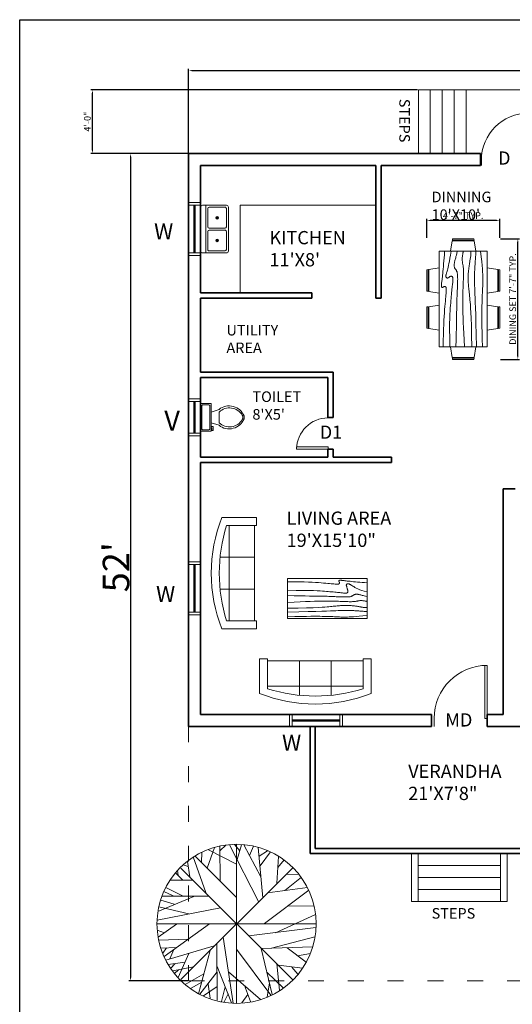
# Model space of a CAD drawing. Units: inches. Extents: x 1662 to 23131, y 1265 to 19127.
# Tile 24 of 26: x 21861 to 22232, y 18361 to 19104. Entities that reach past the tile are written whole.
import ezdxf

# ---------------------------------------------------------------- set-up
doc = ezdxf.new("R2010")
doc.units = ezdxf.units.IN
doc.linetypes.add('ACAD_ISO03W100', pattern=[30, 12, -18])
for name, color, linetype, lineweight in [('A-ANNO-DIMS', 4, 'Continuous', 18), ('A-ANNO-IDEN', 7, 'Continuous', 18), ('A-ANNO-TTLB', 7, 'Continuous', 25), ('A-AREA-IDEN', 7, 'Continuous', 18), ('A-DOOR', 3, 'Continuous', 18), ('A-FLOR-CASE', 8, 'Continuous', 18), ('A-FLOR-FIXT', 9, 'Continuous', 18), ('A-FLOR-STRS', 7, 'Continuous', 18), ('A-FURN', 8, 'Continuous', 18), ('A-GLAZ', 4, 'Continuous', 18), ('A-SITE-PRKG', 8, 'ACAD_ISO03W100', 18), ('A-WALL', 7, 'Continuous', 35), ('L-PLNT', 3, 'Continuous', 18)]:
    doc.layers.add(name, color=color, linetype=linetype, lineweight=lineweight)
doc.styles.get("Standard").update_dxf_attribs({"font": 'arial.ttf'})
doc.dimstyles.new('ISO-25', dxfattribs={"dimtxt": 5, "dimasz": 2.5, "dimexe": 1.25, "dimexo": 0.625, "dimtad": 1, "dimlunit": 3, "dimtxsty": 'Standard', "dimcen": 2.5, "dimadec": 0, "dimazin": 0, "dimtfac": 1, "dimtmove": 0, "dimatfit": 3, "dimfxl": 1, "dimarcsym": 0})

# ---------------------------------------------------------------- blocks, each defined once
blk = doc.blocks.new('*U27')
for p, q in [((0, 0), (0, -6)), ((-40, 0), (-40, -6))]:
    blk.add_line(p, q)
blk.add_lwpolyline([(0, 0), (0, 40), (-1.75, 40), (-1.75, 0)], close=True)
blk.add_arc((0, 0), 40, 90, 180)
blk = doc.blocks.new('*U119')
for p, q in [((-600, 0), (-600, 100)), ((0, 0), (0, 100))]:
    blk.add_line(p, q)
blk.add_lwpolyline([(0, 0), (0, -600), (-43.75, -600), (-43.75, 0)], close=True)
blk.add_arc((0, 0), 600, 180, 270)
blk = doc.blocks.new('*U121')
for p, q in [((0, 0), (0, -100)), ((-900, 0), (-900, -100))]:
    blk.add_line(p, q)
blk.add_lwpolyline([(0, 0), (0, 900), (-43.75, 900), (-43.75, 0)], close=True)
blk.add_arc((0, 0), 900, 90, 180)
blk = doc.blocks.new('Toilet - top')
for p, q in [((9.5, -6), (9.5, -2)), ((-10, -8.5), (-8, -8.5)), ((-10, -9.5), (-10, -8.5)), ((-7, -9.5), (-10, -9.5)), ((-8, -8.5), (-8, -8)), ((-7, -8), (-7, -9.5)), ((-4, -8), (-6, -14)), ((4, -14), (-4, -14)), ((4, -8), (6, -14))]:
    blk.add_line(p, q)
blk.add_lwpolyline([(10.5, -8), (10.5, 0), (-10.5, 0), (-10.5, -8)], close=True)
for points in [[(-9.5, -2), (-9.5, -6)], [(8.5, -1), (-8.5, -1)], [(-8.5, -7), (8.5, -7)]]:
    blk.add_lwpolyline(points)
for centre, radius, start, end in [((-8.62, -1.88), 0.884, 81.8699, 188.1301), ((-8.62, -6.12), 0.884, 171.8699, 278.1301), ((8.62, -1.88), 0.884, 351.8699, 98.1301), ((8.62, -6.12), 0.884, 261.8699, 8.1301), ((3.52, -21.58), 12.17, 141.46911, 247.97143), ((4.2, -21.82), 11.33, 136.36773, 238.94682), ((-3.52, -21.58), 12.17, 292.02843, 38.53071), ((-4.2, -21.82), 11.33, 301.05301, 43.63209), ((0, -27.88), 4, 245.73182, 294.26817), ((0, -29), 4, 254.86053, 285.13947)]:
    blk.add_arc(centre, radius, start, end)
blk = doc.blocks.new('Sink-double - 36 in top')
for p, q in [((-18, -4), (18, -4)), ((-0.75, -18.5), (-0.75, -6.5)), ((0.75, -6.5), (0.75, -18.5))]:
    blk.add_line(p, q)
for points in [[(-16.5, 0), (16.5, 0)], [(-18, -19.5), (-18, -1.5)], [(-16.5, -18.5), (-16.5, -6.5)], [(-15.5, -5.5), (-1.75, -5.5)], [(1.75, -5.5), (15.5, -5.5)], [(16.5, -6.5), (16.5, -18.5)], [(18, -1.5), (18, -19.5)], [(16.5, -21), (-16.5, -21)], [(-1.75, -19.5), (-15.5, -19.5)], [(15.5, -19.5), (1.75, -19.5)]]:
    blk.add_lwpolyline(points)
for centre, radius in [((-8.5, -12.5), 1), ((-8.5, -12.5), 0.5), ((8.5, -12.5), 1), ((8.5, -12.5), 0.5)]:
    blk.add_circle(centre, radius)
for centre, radius, start, end in [((-16.5, -1.5), 1.5, 90, 180), ((16.5, -1.5), 1.5, 0, 90), ((-15.5, -6.5), 1, 90, 180), ((-1.75, -6.5), 1, 0, 90), ((1.75, -6.5), 1, 90, 180), ((15.5, -6.5), 1, 0, 90), ((-16.5, -19.5), 1.5, 180, 270), ((-15.5, -18.5), 1, 180, 270), ((-1.75, -18.5), 1, 270, 0), ((1.75, -18.5), 1, 180, 270), ((15.5, -18.5), 1, 270, 0), ((16.5, -19.5), 1.5, 270, 0)]:
    blk.add_arc(centre, radius, start, end)
blk = doc.blocks.new('Sofa - Roundback 7 ft.')
for p, q in [((-12.00002, -32.4421), (-12.00003, -6.5971)), ((11.99997, -32.4421), (11.99998, -6.5971)), ((-36.000027, -34), (-36.000027, -11.4696)), ((-35.999844, -13.3819), (35.9998, -13.3819)), ((35.99998, -34), (35.99998, -11.4696)), ((-36.000027, -32.4421), (35.99998, -32.4421))]:
    blk.add_line(p, q)
for points in [[(-36.000027, -34), (-42.000027, -34), (-42.000027, -8)], [(41.99998, -8), (41.99998, -34), (35.99998, -34)]]:
    blk.add_lwpolyline(points)
for centre, radius, start, end in [((0, -114.25), 114.25, 68.43141, 111.5686), ((-0.00001, -127.1968), 121.1968, 72.72033, 107.2797)]:
    blk.add_arc(centre, radius, start, end)
blk = doc.blocks.new('Table - Rectangular Woodgrain 60 x 30 in.')
for p, q in [((0, 0), (0, -30)), ((60, 0), (0, 0)), ((60, -30), (60, 0)), ((0, -30), (60, -30))]:
    blk.add_line(p, q)
for points in [[(0, -2.4), (4.8155, -2.418), (9.0302, -2.4688), (12.709, -2.5477), (15.9167, -2.65), (18.7181, -2.7711), (21.1781, -2.9063), (23.3616, -3.0508), (25.3333, -3.2), (27.1477, -3.3495), (28.8172, -3.4958), (30.3437, -3.636), (31.7291, -3.7667), (32.9756, -3.8849), (34.0849, -3.9875), (35.059, -4.0714), (35.9, -4.1334), (36.6114, -4.1711), (37.2041, -4.1854), (37.6906, -4.1779), (38.0833, -4.15), (38.3948, -4.1034), (38.6375, -4.0396), (38.8239, -3.9602), (38.9666, -3.8667), (39.0764, -3.7608), (39.1573, -3.6448), (39.2116, -3.521), (39.2416, -3.3917), (39.2498, -3.2593), (39.2385, -3.1261), (39.21, -2.9944), (39.1666, -2.8667), (39.111, -2.7447), (39.0468, -2.6281), (38.978, -2.5163), (38.9083, -2.4083), (38.8418, -2.3035), (38.7823, -2.201), (38.7337, -2.1001), (38.7, -2), (38.6844, -1.9003), (38.6875, -1.8021), (38.7094, -1.707), (38.75, -1.6167), (38.8094, -1.5326), (38.8875, -1.4563), (38.9844, -1.3893), (39.1, -1.3333), (39.2351, -1.2896), (39.3937, -1.2583), (39.5804, -1.2396), (39.8, -1.2333), (40.057, -1.2396), (40.3562, -1.2583), (40.7023, -1.2896), (41.1, -1.3333), (41.5547, -1.3895), (42.0755, -1.4573), (42.6721, -1.5361), (43.3542, -1.625), (44.1316, -1.7233), (45.014, -1.8302), (46.0114, -1.9449), (47.1333, -2.0667), (48.3862, -2.1947), (49.7625, -2.3281), (51.2513, -2.4663), (52.8416, -2.6083), (54.5226, -2.7535), (56.2833, -2.9011), (58.1127, -3.0501), (60, -3.2)], [(0, -9.2), (6.5759, -9.0858), (11.9385, -9.0365), (16.2527, -9.0418), (19.6833, -9.0917), (22.3952, -9.1759), (24.5531, -9.2844), (26.322, -9.4069), (27.8666, -9.5333), (29.3241, -9.6553), (30.7203, -9.7719), (32.0532, -9.8837), (33.3208, -9.9917), (34.5213, -10.0965), (35.6526, -10.199), (36.7128, -10.2999), (37.7, -10.4), (38.6129, -10.4996), (39.4531, -10.5969), (40.223, -10.6895), (40.925, -10.775), (41.5613, -10.8512), (42.1344, -10.9156), (42.6465, -10.966), (43.1, -11), (43.4976, -11.0158), (43.8437, -11.0136), (44.143, -10.9942), (44.4, -10.9583), (44.6195, -10.9069), (44.8062, -10.8406), (44.9648, -10.7603), (45.1, -10.6667), (45.2155, -10.5598), (45.3114, -10.4365), (45.3871, -10.2929), (45.4416, -10.125), (45.4743, -9.929), (45.4844, -9.7011), (45.4709, -9.4371), (45.4333, -9.1333), (45.3716, -8.7883), (45.2896, -8.4104), (45.1919, -8.0107), (45.0833, -7.6), (44.9685, -7.1893), (44.8521, -6.7896), (44.7388, -6.4117), (44.6333, -6.0667), (44.54, -5.7628), (44.4614, -5.4979), (44.4001, -5.2675), (44.3583, -5.0667), (44.3384, -4.8909), (44.3427, -4.7354), (44.3736, -4.5956), (44.4333, -4.4667), (44.5236, -4.3453), (44.6427, -4.2333), (44.7884, -4.1339), (44.9583, -4.05), (45.1501, -3.9849), (45.3614, -3.9417), (45.59, -3.9234), (45.8333, -3.9333), (46.0915, -3.9749), (46.3734, -4.0531), (46.6906, -4.1736), (47.0542, -4.3417), (47.4756, -4.5629), (47.9661, -4.8427), (48.5372, -5.1866), (49.2, -5.6), (49.9676, -6.0844), (50.8594, -6.625), (51.8965, -7.2031), (53.1, -7.8), (54.491, -8.3969), (56.0906, -8.975), (57.9199, -9.5156), (60, -10)], [(0, -12.8), (5.1847, -12.9322), (9.6213, -13.0323), (13.3963, -13.1059), (16.5958, -13.1583), (19.3063, -13.1952), (21.614, -13.2219), (23.6054, -13.2439), (25.3666, -13.2667), (26.9728, -13.2947), (28.4531, -13.3281), (29.8256, -13.3663), (31.1083, -13.4083), (32.3191, -13.4535), (33.476, -13.501), (34.597, -13.5501), (35.7, -13.6), (36.7984, -13.6497), (37.8875, -13.6979), (38.9578, -13.743), (40, -13.7833), (41.0047, -13.8174), (41.9625, -13.8438), (42.864, -13.8607), (43.7, -13.8667), (44.4631, -13.8604), (45.1552, -13.8417), (45.7801, -13.8104), (46.3416, -13.7667), (46.8439, -13.7104), (47.2906, -13.6417), (47.6858, -13.5604), (48.0333, -13.4667), (48.3375, -13.3608), (48.6042, -13.2448), (48.8396, -13.121), (49.05, -12.9917), (49.2417, -12.8593), (49.4208, -12.7261), (49.5937, -12.5944), (49.7667, -12.4667), (49.9452, -12.3451), (50.1323, -12.2313), (50.3303, -12.1268), (50.5416, -12.0333), (50.7686, -11.9524), (51.0135, -11.8854), (51.2788, -11.8341), (51.5666, -11.8), (51.8785, -11.7843), (52.2116, -11.7865), (52.562, -11.8059), (52.926, -11.8417), (53.2998, -11.8931), (53.6795, -11.9594), (54.0614, -12.0397), (54.4416, -12.1333), (54.8223, -12.2401), (55.2293, -12.3625), (55.6942, -12.5037), (56.2489, -12.6667), (56.9251, -12.8547), (57.7545, -13.0708), (58.7689, -13.3182), (60, -13.6)], [(0, -18), (5.124, -17.7273), (9.6609, -17.5057), (13.6705, -17.3303), (17.2125, -17.1958), (20.3467, -17.0973), (23.1328, -17.0297), (25.6307, -16.9878), (27.9, -16.9667), (29.9928, -16.9617), (31.9302, -16.9703), (33.7254, -16.9907), (35.3917, -17.0208), (36.9423, -17.0588), (38.3906, -17.1026), (39.7499, -17.1503), (41.0333, -17.2), (42.2519, -17.2496), (43.4073, -17.2969), (44.4986, -17.3395), (45.525, -17.375), (46.4858, -17.4012), (47.3802, -17.4156), (48.2074, -17.416), (48.9667, -17.4), (49.6583, -17.3662), (50.2872, -17.3167), (50.8595, -17.2547), (51.3812, -17.1833), (51.8584, -17.1057), (52.2971, -17.025), (52.7034, -16.9443), (53.0833, -16.8667), (53.443, -16.7951), (53.789, -16.7313), (54.128, -16.6768), (54.4666, -16.6334), (54.8115, -16.6024), (55.1693, -16.5854), (55.5465, -16.5841), (55.95, -16.6), (56.3828, -16.6337), (56.8346, -16.6823), (57.2915, -16.7418), (57.7396, -16.8084), (58.165, -16.878), (58.5539, -16.9469), (58.8924, -17.0111), (59.1666, -17.0667), (59.3679, -17.1107), (59.5078, -17.1438), (59.6032, -17.1675), (59.6708, -17.1833), (59.7275, -17.193), (59.7901, -17.1979), (59.8753, -17.1998), (60, -17.2)], [(0, -22.4), (8.0098, -22.2501), (14.4094, -22.1011), (19.4168, -21.9535), (23.25, -21.8083), (26.1269, -21.6663), (28.2656, -21.5281), (29.884, -21.3947), (31.2, -21.2667), (32.3967, -21.1448), (33.5172, -21.0292), (34.5697, -20.9198), (35.5625, -20.8167), (36.5037, -20.7198), (37.4015, -20.6292), (38.2642, -20.5448), (39.1, -20.4667), (39.9164, -20.3951), (40.7187, -20.3313), (41.5117, -20.2768), (42.3, -20.2333), (43.0883, -20.2024), (43.8812, -20.1854), (44.6836, -20.1841), (45.5, -20.2), (46.3328, -20.234), (47.1747, -20.2844), (48.0163, -20.3488), (48.8479, -20.425), (49.66, -20.5106), (50.4429, -20.6031), (51.1872, -20.7004), (51.8833, -20.8), (52.5246, -20.8999), (53.1166, -20.9995), (53.6681, -21.0983), (54.1875, -21.1958), (54.6834, -21.2919), (55.1646, -21.3859), (55.6394, -21.4777), (56.1167, -21.5667), (56.6028, -21.6515), (57.0961, -21.7266), (57.5929, -21.7852), (58.0896, -21.8208), (58.5823, -21.8268), (59.0674, -21.7964), (59.5412, -21.723), (60, -21.6)], [(0, -25.2), (8.6355, -25.0504), (15.7026, -24.9031), (21.4049, -24.7606), (25.9458, -24.625), (29.529, -24.4988), (32.3578, -24.3844), (34.6359, -24.284), (36.5667, -24.2), (38.3213, -24.1341), (39.9417, -24.0854), (41.437, -24.0523), (42.8167, -24.0333), (44.0901, -24.0268), (45.2667, -24.0313), (46.3557, -24.0451), (47.3667, -24.0667), (48.309, -24.0947), (49.1928, -24.1287), (50.0284, -24.168), (50.826, -24.2125), (51.5959, -24.2617), (52.3483, -24.3151), (53.0935, -24.3725), (53.8417, -24.4334), (54.6009, -24.497), (55.3699, -24.561), (56.1454, -24.6226), (56.9239, -24.6792), (57.7021, -24.7279), (58.4764, -24.7662), (59.2435, -24.7911), (60, -24.8)], [(0, -28.8), (5.6867, -28.6681), (10.45, -28.5698), (14.407, -28.5012), (17.675, -28.4584), (20.3711, -28.4374), (22.6125, -28.4344), (24.5164, -28.4455), (26.2, -28.4667), (27.762, -28.4947), (29.2276, -28.5281), (30.6033, -28.5663), (31.8958, -28.6084), (33.1118, -28.6535), (34.2578, -28.7011), (35.3405, -28.7501), (36.3666, -28.8), (37.3443, -28.8497), (38.288, -28.8974), (39.2137, -28.9412), (40.1375, -28.9792), (41.0753, -29.0093), (42.0432, -29.0297), (43.0572, -29.0384), (44.1333, -29.0333), (45.2936, -29.0114), (46.5843, -28.9641), (48.0579, -28.8816), (49.7666, -28.7542), (51.7629, -28.5721), (54.0989, -28.3255), (56.8272, -28.0048), (60, -27.6)]]:
    blk.add_lwpolyline(points)
blk = doc.blocks.new('Dining Set - 36 x 72 in.')
for p, q in [((-22.2343, 26.00059), (-23.4847, 17.99762)), ((-22.2304, 26), (-5.7608, 26)), ((-22, 27.5), (-22.1562, 26.50042)), ((-5.8416, 26.5), (-22.1534, 26.5)), ((-22, 27.5), (-6, 27.5)), ((-5.8437, 26.49966), (-6, 27.5)), ((-4.5152, 17.99762), (-5.7655, 25.99926)), ((5.7657, 26.00059), (4.5153, 17.99762)), ((5.7696, 26), (22.2392, 26)), ((6, 27.5), (5.8438, 26.50042)), ((22.1584, 26.5), (5.8466, 26.5)), ((6, 27.5), (22, 27.5)), ((22.1563, 26.49966), (22, 27.5)), ((23.4848, 17.99762), (22.2345, 25.99926)), ((36, 18), (-36, 18)), ((-36, 18), (-36, -18)), ((36, -18), (36, 18)), ((-45.5, 8), (-44.5004, 8.15617)), ((-45.5, 8), (-45.5, -8)), ((-44.5, -8.15843), (-44.5, 8.15338)), ((-44.0006, 8.23428), (-35.9976, 9.48474)), ((-44, 8.23041), (-44, -8.23915)), ((44.0006, 8.23428), (35.9976, 9.48474)), ((44, 8.23041), (44, -8.23915)), ((44.5, -8.15843), (44.5, 8.15338)), ((45.5, 8), (44.5005, 8.15617)), ((45.5, 8), (45.5, -8)), ((-44.4997, -8.15631), (-45.5, -8)), ((-35.9976, -9.48476), (-43.9993, -8.2345)), ((35.9976, -9.48476), (43.9993, -8.2345)), ((44.4997, -8.15631), (45.5, -8)), ((-36, -18), (36, -18)), ((-22.2343, -26.0006), (-23.4847, -17.99762)), ((-4.5152, -17.99762), (-5.7655, -25.99928)), ((5.7657, -26.0006), (4.5153, -17.99762)), ((23.4848, -17.99762), (22.2345, -25.99928)), ((-22.2304, -26), (-5.7608, -26)), ((-22, -27.5), (-22.1562, -26.50044)), ((-5.8416, -26.5), (-22.1534, -26.5)), ((-22, -27.5), (-6, -27.5)), ((-5.8437, -26.49967), (-6, -27.5)), ((5.7696, -26), (22.2392, -26)), ((6, -27.5), (5.8438, -26.50044)), ((22.1584, -26.5), (5.8466, -26.5)), ((6, -27.5), (22, -27.5)), ((22.1563, -26.49967), (22, -27.5))]:
    blk.add_line(p, q)
for points in [[(-36, 15), (-31.1772, 14.97754), (-26.8079, 14.91406), (-22.8538, 14.81543), (-19.276, 14.6875), (-16.0362, 14.53613), (-13.0957, 14.36718), (-10.4159, 14.18652), (-7.9583, 14), (-5.6904, 13.81315), (-3.6035, 13.63021), (-1.6954, 13.45508), (0.0365, 13.29166), (1.5945, 13.14388), (2.9811, 13.01562), (4.1988, 12.9108), (5.25, 12.83333), (6.1393, 12.78613), (6.8802, 12.76823), (7.4883, 12.77767), (7.9792, 12.8125), (8.3685, 12.87077), (8.6719, 12.95052), (8.9049, 13.0498), (9.0833, 13.16666), (9.2205, 13.29899), (9.3216, 13.44401), (9.3895, 13.59879), (9.4271, 13.76041), (9.4373, 13.92594), (9.4232, 14.09245), (9.3875, 14.257), (9.3333, 14.41666), (9.2638, 14.56917), (9.1836, 14.71484), (9.0975, 14.85465), (9.0104, 14.98958), (8.9272, 15.1206), (8.8529, 15.2487), (8.7922, 15.37483), (8.75, 15.5), (8.7305, 15.62467), (8.7344, 15.74739), (8.7617, 15.86621), (8.8125, 15.97916), (8.8867, 16.08431), (8.9844, 16.17968), (9.1055, 16.26334), (9.25, 16.33333), (9.4189, 16.38802), (9.6172, 16.42708), (9.8506, 16.45052), (10.125, 16.45833), (10.4463, 16.45052), (10.8203, 16.42708), (11.2529, 16.38802), (11.75, 16.33333), (12.3184, 16.26318), (12.9694, 16.17838), (13.7151, 16.07991), (14.5677, 15.96875), (15.5395, 15.84586), (16.6426, 15.71224), (17.8893, 15.56884), (19.2917, 15.41666), (20.859, 15.25667), (22.5879, 15.08984), (24.4721, 14.91715), (26.5052, 14.73958), (28.6809, 14.5581), (30.9929, 14.3737), (33.4347, 14.18733), (36, 14)], [(-36, 10), (-28.9766, 10.14274), (-23.1725, 10.20442), (-18.4241, 10.19775), (-14.5677, 10.13541), (-11.4399, 10.03011), (-8.877, 9.89453), (-6.7154, 9.74137), (-4.7917, 9.58333), (-2.9698, 9.43082), (-1.2246, 9.28515), (0.4415, 9.14534), (2.026, 9.01041), (3.5266, 8.87939), (4.9408, 8.7513), (6.266, 8.62516), (7.5, 8.5), (8.6411, 8.37549), (9.6914, 8.2539), (10.6538, 8.13818), (11.5312, 8.03125), (12.3267, 7.93603), (13.043, 7.85547), (13.6831, 7.79248), (14.25, 7.75), (14.7471, 7.7303), (15.1797, 7.73307), (15.5537, 7.75732), (15.875, 7.80208), (16.1494, 7.86637), (16.3828, 7.94922), (16.5811, 8.04964), (16.75, 8.16666), (16.8944, 8.29915), (17.0143, 8.44531), (17.1089, 8.60319), (17.1771, 8.77083), (17.218, 8.94629), (17.2305, 9.1276), (17.2137, 9.31282), (17.1667, 9.5), (17.0895, 9.6875), (16.987, 9.875), (16.8649, 10.0625), (16.7292, 10.25), (16.5856, 10.4375), (16.4401, 10.625), (16.2985, 10.8125), (16.1667, 11), (16.05, 11.18733), (15.9518, 11.3737), (15.8752, 11.5581), (15.8229, 11.73958), (15.798, 11.91715), (15.8034, 12.08984), (15.842, 12.25667), (15.9167, 12.41666), (16.0295, 12.56836), (16.1784, 12.70833), (16.3605, 12.83268), (16.5729, 12.9375), (16.8127, 13.01888), (17.0768, 13.07291), (17.3625, 13.0957), (17.6667, 13.08333), (17.9894, 13.03312), (18.3418, 12.94726), (18.7382, 12.82918), (19.1927, 12.68229), (19.7195, 12.51001), (20.3327, 12.31575), (21.0465, 12.10294), (21.875, 11.875), (22.8357, 11.63354), (23.959, 11.37304), (25.2786, 11.08618), (26.8282, 10.76562), (28.6414, 10.40405), (30.752, 9.99414), (33.1936, 9.52856), (36, 9)], [(-36, 5.5), (-30.7157, 5.3348), (-26.069, 5.20963), (-21.9946, 5.11767), (-18.4271, 5.05208), (-15.3009, 5.00602), (-12.5508, 4.97265), (-10.1112, 4.94515), (-7.9167, 4.91666), (-5.909, 4.88167), (-4.0586, 4.83984), (-2.3429, 4.79215), (-0.7396, 4.73958), (0.7739, 4.6831), (2.22, 4.6237), (3.6213, 4.56233), (5, 4.5), (6.373, 4.43782), (7.7344, 4.3776), (9.0723, 4.32129), (10.375, 4.27083), (11.6309, 4.22819), (12.8281, 4.19531), (13.9551, 4.17415), (15, 4.16666), (15.954, 4.17448), (16.819, 4.19791), (17.6001, 4.23698), (18.3021, 4.29166), (18.9299, 4.36198), (19.4883, 4.44791), (19.9823, 4.54948), (20.4167, 4.66666), (20.7969, 4.79899), (21.1302, 4.94401), (21.4245, 5.09879), (21.6875, 5.26041), (21.9271, 5.42594), (22.1511, 5.59245), (22.3672, 5.757), (22.5834, 5.91666), (22.8065, 6.06868), (23.0404, 6.21093), (23.2879, 6.34147), (23.5521, 6.45833), (23.8358, 6.55957), (24.142, 6.64323), (24.4735, 6.70735), (24.8334, 6.75), (25.2235, 6.76969), (25.642, 6.76692), (26.0858, 6.74267), (26.5521, 6.69791), (27.0379, 6.63362), (27.5404, 6.55078), (28.0565, 6.45036), (28.5834, 6.33333), (29.1242, 6.19987), (29.7071, 6.04687), (30.3661, 5.87044), (31.1354, 5.66666), (32.0493, 5.43164), (33.142, 5.16146), (34.4475, 4.85221), (36, 4.5)], [(-36, -1), (-30.7915, -0.6591), (-26.0195, -0.38216), (-21.6519, -0.16284), (-17.6563, 0.00521), (-14.0005, 0.12833), (-10.6523, 0.21289), (-7.5796, 0.26522), (-4.75, 0.29166), (-2.134, 0.29793), (0.2878, 0.28711), (2.5317, 0.26163), (4.6146, 0.22396), (6.5529, 0.17651), (8.3633, 0.12174), (10.0623, 0.06209), (11.6667, 0), (13.1899, -0.06201), (14.6341, -0.1211), (15.9982, -0.17432), (17.2813, -0.21875), (18.4823, -0.25147), (19.6003, -0.26953), (20.6343, -0.27002), (21.5834, -0.25), (22.4481, -0.20768), (23.2357, -0.14584), (23.9549, -0.06836), (24.6146, 0.02083), (25.2235, 0.11784), (25.7904, 0.21875), (26.3241, 0.31966), (26.8334, 0.41666), (27.3265, 0.50618), (27.8099, 0.58593), (28.2894, 0.65397), (28.7709, 0.70833), (29.2601, 0.74707), (29.763, 0.76823), (30.2855, 0.76985), (30.8334, 0.75), (31.4088, 0.70784), (31.9994, 0.64713), (32.589, 0.57275), (33.1615, 0.48958), (33.7008, 0.4025), (34.1908, 0.3164), (34.6153, 0.23616), (34.9584, 0.16666), (35.2099, 0.11165), (35.3848, 0.07031), (35.504, 0.04069), (35.5886, 0.02083), (35.6594, 0.00879), (35.7377, 0.0026), (35.8442, 0.00032), (36, 0)], [(-36, -6.5), (-27.1843, -6.31267), (-20.084, -6.1263), (-14.469, -5.9419), (-10.1094, -5.76042), (-6.7752, -5.58285), (-4.2363, -5.41016), (-2.2629, -5.24333), (-0.625, -5.08334), (0.8708, -4.93099), (2.2715, -4.78646), (3.5872, -4.64974), (4.8281, -4.52084), (6.0046, -4.39974), (7.127, -4.28646), (8.2053, -4.18099), (9.25, -4.08334), (10.2705, -3.99382), (11.2734, -3.91407), (12.2647, -3.84603), (13.25, -3.79167), (14.2354, -3.75293), (15.2266, -3.73177), (16.2295, -3.73015), (17.25, -3.75), (18.2912, -3.79248), (19.3451, -3.85547), (20.4009, -3.93604), (21.4479, -4.03125), (22.4754, -4.13819), (23.4727, -4.25391), (24.4289, -4.37549), (25.3334, -4.5), (26.1785, -4.62492), (26.9694, -4.74935), (27.7145, -4.87281), (28.4219, -4.99479), (29.1, -5.11483), (29.7572, -5.23242), (30.4016, -5.34709), (31.0417, -5.45834), (31.6837, -5.56437), (32.3262, -5.65821), (32.9658, -5.73153), (33.599, -5.77604), (34.2224, -5.78345), (34.8327, -5.74545), (35.4264, -5.65373), (36, -5.5)], [(-36, -10), (-26.4022, -9.81299), (-18.4675, -9.62891), (-11.9839, -9.45069), (-6.7396, -9.28125), (-2.5226, -9.12354), (0.8789, -8.98047), (3.6769, -8.85498), (6.0833, -8.75), (8.2767, -8.66765), (10.3021, -8.60677), (12.1712, -8.56543), (13.8958, -8.54167), (15.4876, -8.53353), (16.9583, -8.53907), (18.3197, -8.55632), (19.5834, -8.58334), (20.7616, -8.61841), (21.8685, -8.66081), (22.9188, -8.71004), (23.9271, -8.76563), (24.9081, -8.82707), (25.8763, -8.89388), (26.8465, -8.96558), (27.8334, -9.04167), (28.8474, -9.12118), (29.8828, -9.20117), (30.93, -9.27824), (31.9792, -9.34896), (33.0205, -9.40991), (34.0443, -9.45768), (35.0407, -9.48885), (36, -9.5)], [(-36, -14.5), (-30.0881, -14.33513), (-25.0332, -14.21224), (-20.7312, -14.12647), (-17.0781, -14.07292), (-13.97, -14.04671), (-11.3027, -14.04297), (-8.9724, -14.05681), (-6.875, -14.08334), (-4.9224, -14.11833), (-3.0905, -14.16016), (-1.3709, -14.20785), (0.2448, -14.26042), (1.7647, -14.3169), (3.1973, -14.3763), (4.5507, -14.43767), (5.8333, -14.5), (7.0554, -14.5621), (8.235, -14.62175), (9.3922, -14.67652), (10.5469, -14.72396), (11.7192, -14.76164), (12.929, -14.78711), (14.1965, -14.79794), (15.5417, -14.79167), (16.9933, -14.76424), (18.6152, -14.70508), (20.4804, -14.60197), (22.6615, -14.44271), (25.2312, -14.21509), (28.2624, -13.9069), (31.8277, -13.50594), (36, -13)]]:
    blk.add_lwpolyline(points)
blk = doc.blocks.new('*D122')
at = {"layer": 'A-ANNO-DIMS', "color": 0, "lineweight": -2, "transparency": 16777216}
for p, q in [((21987.52, 19002.71), (21943.13, 19002.71)), ((21944.38, 19000.21), (21944.38, 18381.21)), ((21987.52, 18378.71), (21943.13, 18378.71))]:
    blk.add_line(p, q, dxfattribs=at)
at = {"layer": 'A-ANNO-DIMS', "color": 0, "transparency": 16777216}
for points in [[(21943.97, 19000.21), (21944.8, 19000.21), (21944.38, 19002.71)], [(21943.97, 18381.21), (21944.8, 18381.21), (21944.38, 18378.71)]]:
    blk.add_solid(points, dxfattribs=at)
at = {"layer": 'Defpoints', "color": 0, "transparency": 16777216}
for p in [(21988.15, 19002.71), (21944.38, 18378.71), (21988.15, 18378.71)]:
    blk.add_point(p, dxfattribs=at)
at = {"layer": 'A-ANNO-DIMS', "color": 0, "transparency": 16777216, "insert": (21933.55, 18690.71), "char_height": 5, "attachment_point": 5, "rotation": 90}
blk.add_mtext("{\\H4x;52'}", dxfattribs=at)
blk = doc.blocks.new('*D124')
at = {"layer": 'A-ANNO-DIMS', "color": 0, "lineweight": -2, "transparency": 16777216}
for p, q in [((21988.15, 19003.33), (21988.15, 19066.63)), ((21990.65, 19065.38), (22537.65, 19065.38)), ((22540.15, 19003.33), (22540.15, 19066.63))]:
    blk.add_line(p, q, dxfattribs=at)
at = {"layer": 'A-ANNO-DIMS', "color": 0, "transparency": 16777216}
for points in [[(21990.65, 19065.79), (21990.65, 19064.96), (21988.15, 19065.38)], [(22537.65, 19065.79), (22537.65, 19064.96), (22540.15, 19065.38)]]:
    blk.add_solid(points, dxfattribs=at)
at = {"layer": 'Defpoints', "color": 0, "transparency": 16777216}
for p in [(22540.15, 19065.38), (21988.15, 19002.71), (22540.15, 19002.71)]:
    blk.add_point(p, dxfattribs=at)
at = {"layer": 'A-ANNO-DIMS', "color": 0, "transparency": 16777216, "insert": (22264.15, 19076.21), "char_height": 5, "attachment_point": 5}
blk.add_mtext("{\\H4x;46'}", dxfattribs=at)
blk = doc.blocks.new('*U133')
for p, q in [((-318.48552, 1395.49124), (-202.21702, 1510.14684)), ((-135.1407, 1515.88724), (419.3667, 426.62602)), ((61.6204, 1395.49124), (-36.75888, 1521.60224)), ((0, 1523.98984), (0, -1524)), ((12.43076, 1234.96832), (92.92336, 1515.88724)), ((464.08594, 902.45692), (137.6426, 1515.88724)), ((-671.75888, 1183.37076), (-667.28848, 1366.81464)), ((-559.96332, 1068.71262), (-421.33774, 1464.27444)), ((-537.60624, 1418.42744), (-0.98552, 1143.23876)), ((-314.01258, 816.46522), (-318.48552, 1492.95104)), ((249.43562, 1309.49446), (325.45782, 1487.21064)), ((499.8593, 495.41938), (414.89376, 1464.27444)), ((432.78298, 1298.0289), (589.29524, 1401.23164)), ((450.66966, 1108.84208), (647.43076, 1378.29544)), ((-1020.56438, 1131.7732), (-926.6555, 1097.37652)), ((-940.07178, 1194.83632), (-895.35, 902.45692)), ((-828.27368, 1280.83056), (-591.26628, 598.61196)), ((-792.50032, 1298.0289), (-5.45846, 512.61772)), ((803.94302, 1292.29612), (768.16966, 776.33322)), ((790.52928, 1080.17818), (911.26818, 1223.50022)), ((-1163.66036, 971.25282), (-1029.50772, 839.39634)), ((-1114.47072, 925.38804), (-1127.887, 1022.84784)), ((1066.8, 1066.8), (-1066.8, -1066.8)), ((1066.8, -1066.8), (-1066.8, 1066.8)), ((942.57114, 942.58892), (1184.04894, 954.05448)), ((-1266.51258, 833.66356), (-832.74662, 833.66356)), ((920.21152, 638.74396), (1242.18446, 890.99136)), ((-1391.72442, 621.54308), (-1212.85, 535.55138)), ((-1351.47812, 696.07176), (-1020.56438, 529.8186)), ((1380.81004, 644.47674), (531.16226, 8.12292)), ((593.76818, 592.87918), (1353.98002, 696.07176)), ((-819.33034, 524.08582), (-1503.51998, 237.4392)), ((-1449.8574, 455.28992), (-1194.96332, 375.02846)), ((-1423.02738, 529.8186), (-528.66036, 529.8186)), ((-1516.93626, 71.1835), (-305.06924, 306.2351)), ((-1490.10624, 323.43344), (-913.23922, 191.57696)), ((978.3445, 340.63178), (1479.19186, 346.36456)), ((-1387.25148, -628.2309), (-515.24662, 2.39014)), ((745.81004, -169.59834), (1510.49228, 180.1114)), ((-1524, 0), (1524, 0)), ((-1516.93626, -123.73356), (-1378.30814, -169.59834)), ((-1150.24662, -3.34264), (-1499.04958, -255.59258)), ((236.02188, -232.65892), (1514.96522, -72.13854)), ((-1485.6333, -312.92038), (-926.6555, -295.72204)), ((-255.8796, -255.59258), (-63.59144, -1516.83212)), ((669.79038, -467.71052), (1497.07854, -249.85726)), ((-1449.8574, -467.71052), (-1150.24662, -456.24496)), ((-1338.06438, -461.9752), (-1409.61364, -559.43754)), ((-1351.47812, -697.0268), (-425.80814, -421.84574)), ((-1199.43626, -490.64164), (-1275.45592, -668.3629)), ((-506.30074, -513.57276), (-725.42146, -1339.1134)), ((-376.6185, -381.71628), (-372.1481, -1465.2371)), ((-0.98552, -484.90886), (656.3741, -1367.7773)), ((473.02928, -473.44076), (678.73372, -1356.31174)), ((477.49968, -473.44076), (1456.83224, -439.04662)), ((969.40116, -461.9752), (1331.6204, -737.15626)), ((1166.16226, -611.03256), (1412.113, -565.17032)), ((-989.25888, -737.15626), (-1306.75888, -777.28572)), ((-913.23922, -570.9031), (-1118.94366, -1029.53566)), ((-1181.54958, -765.82016), (-1257.56924, -851.8144)), ((-823.80074, -823.1505), (-1221.79334, -903.41196)), ((-1110.00032, -880.4783), (-1186.01998, -949.2742)), ((-372.1481, -920.6103), (-703.06438, -1344.84618)), ((-372.1481, -817.41772), (-99.3648, -1511.10188)), ((-157.50032, -920.6103), (455.1426, -1448.03876)), ((580.3519, -926.34308), (897.8519, -1230.18804)), ((772.6426, -765.82016), (821.83224, -1270.3175)), ((799.47262, -794.4866), (1260.07114, -846.08162)), ((1054.3667, -828.88328), (1170.6352, -966.47254)), ((-627.04218, -960.73976), (-984.78848, -1161.39214)), ((-667.28848, -1115.5299), (-881.93626, -1235.92082)), ((-372.1481, -1201.52414), (-635.98552, -1379.24286)), ((-546.54958, -1155.65936), (-506.30074, -1425.1051)), ((-215.6333, -1207.25692), (-291.6555, -1488.16822)), ((151.05634, -1184.32326), (267.32484, -1488.16822)), ((629.54408, -1138.46102), (584.82484, -1396.4412)), ((-161.97072, -1339.1134), (-237.99292, -1493.901)), ((213.66226, -1350.57896), (97.39376, -1511.10188))]:
    blk.add_line(p, q)
blk.add_circle((0, 0), 1524)
blk = doc.blocks.new('VENT-24-J9X2')
for p, q in [((9, 28), (0, 28)), ((9, 26), (0, 26)), ((4, 26), (4, 2)), ((4.5, 26), (4.5, 2)), ((5, 26), (5, 2)), ((9, 2), (0, 2)), ((9, 0), (0, 0))]:
    blk.add_line(p, q)
blk = doc.blocks.new('WIN-36-J9X2')
for p, q in [((0, 0), (0, 9)), ((2, 0), (2, 9)), ((38, 0), (38, 9)), ((40, 0), (40, 9)), ((38, 5), (2, 5)), ((38, 4.5), (2, 4.5)), ((38, 4), (2, 4))]:
    blk.add_line(p, q)
blk = doc.blocks.new('*D177')
at = {"layer": 'A-ANNO-DIMS', "color": 0, "lineweight": -2, "transparency": 16777216}
for p, q in [((22223.17, 18938.46), (22237.45, 18938.46)), ((22236.2, 18849.96), (22236.2, 18935.96)), ((22223.17, 18847.46), (22237.45, 18847.46))]:
    blk.add_line(p, q, dxfattribs=at)
at = {"layer": 'A-ANNO-DIMS', "color": 0, "transparency": 16777216}
for points in [[(22235.78, 18935.96), (22236.62, 18935.96), (22236.2, 18938.46)], [(22235.78, 18849.96), (22236.62, 18849.96), (22236.2, 18847.46)]]:
    blk.add_solid(points, dxfattribs=at)
at = {"layer": 'Defpoints', "color": 0, "transparency": 16777216}
for p in [(22222.55, 18938.46), (22236.2, 18938.46), (22222.55, 18847.46)]:
    blk.add_point(p, dxfattribs=at)
at = {"layer": 'A-ANNO-DIMS', "color": 0, "transparency": 16777216, "insert": (22232.99, 18892.96), "char_height": 5, "attachment_point": 5, "rotation": 90}
blk.add_mtext('DINING SET 7\'-7" TYP.', dxfattribs=at)
blk = doc.blocks.new('*D178')
at = {"layer": 'A-ANNO-DIMS', "color": 0, "lineweight": -2, "transparency": 16777216}
for p, q in [((22167.55, 18939.08), (22167.55, 18953.36)), ((22220.05, 18952.11), (22170.05, 18952.11)), ((22222.55, 18939.08), (22222.55, 18953.36))]:
    blk.add_line(p, q, dxfattribs=at)
at = {"layer": 'A-ANNO-DIMS', "color": 0, "transparency": 16777216}
for points in [[(22170.05, 18952.52), (22170.05, 18951.69), (22167.55, 18952.11)], [(22220.05, 18952.52), (22220.05, 18951.69), (22222.55, 18952.11)]]:
    blk.add_solid(points, dxfattribs=at)
at = {"layer": 'Defpoints', "color": 0, "transparency": 16777216}
for p in [(22167.55, 18952.11), (22167.55, 18938.46), (22222.55, 18938.46)]:
    blk.add_point(p, dxfattribs=at)
at = {"layer": 'A-ANNO-DIMS', "color": 0, "transparency": 16777216, "insert": (22195.05, 18955.23), "char_height": 5, "attachment_point": 5}
blk.add_mtext('4\'-7" TYP.', dxfattribs=at)
blk = doc.blocks.new('*D254')
at = {"layer": 'A-ANNO-DIMS', "color": 0, "lineweight": -2, "transparency": 16777216}
for p, q in [((22160.65, 19050.71), (21914.55, 19050.71)), ((21915.8, 19005.21), (21915.8, 19048.21)), ((22160.65, 19002.71), (21914.55, 19002.71))]:
    blk.add_line(p, q, dxfattribs=at)
at = {"layer": 'A-ANNO-DIMS', "color": 0, "transparency": 16777216}
for points in [[(21915.38, 19048.21), (21916.21, 19048.21), (21915.8, 19050.71)], [(21915.38, 19005.21), (21916.21, 19005.21), (21915.8, 19002.71)]]:
    blk.add_solid(points, dxfattribs=at)
at = {"layer": 'Defpoints', "color": 0, "transparency": 16777216}
for p in [(21915.8, 19050.71), (22161.27, 19050.71), (22161.27, 19002.71)]:
    blk.add_point(p, dxfattribs=at)
at = {"layer": 'A-ANNO-DIMS', "color": 0, "transparency": 16777216, "insert": (21912.62, 19026.71), "char_height": 5, "attachment_point": 5, "rotation": 90}
blk.add_mtext('4\'-0"', dxfattribs=at)

msp = doc.modelspace()

# ---------------------------------------------------------------- linework, layer by layer
at = {"layer": 'A-ANNO-TTLB'}
msp.add_lwpolyline([(21860.989, 19103.605), (23130.86, 19103.605), (23130.86, 17867.351), (21860.989, 17867.351)], close=True, dxfattribs=at)
at = {"layer": 'A-FLOR-CASE'}
for p, q in [((22027.149, 18963.71), (22129.149, 18963.71)), ((22027.149, 18897.71), (22027.149, 18963.71))]:
    msp.add_line(p, q, dxfattribs=at)
at = {"layer": 'A-FLOR-STRS'}
for p, q in [((22257.149, 19050.71), (22161.274, 19050.71)), ((22161.274, 19050.71), (22161.274, 19002.71)), ((22170.274, 19050.71), (22170.274, 19002.71)), ((22179.274, 19050.71), (22179.274, 19002.71)), ((22188.274, 19050.71), (22188.274, 19002.71)), ((22197.274, 19050.71), (22197.274, 19002.71)), ((22156.149, 18474.71), (22156.149, 18438.71)), ((22161.149, 18474.71), (22161.149, 18438.71)), ((22223.149, 18474.71), (22223.149, 18438.71)), ((22228.149, 18474.71), (22228.149, 18438.71)), ((22223.149, 18465.71), (22161.149, 18465.71)), ((22223.149, 18456.71), (22161.149, 18456.71)), ((22223.149, 18447.71), (22161.149, 18447.71)), ((22228.149, 18438.71), (22156.149, 18438.71))]:
    msp.add_line(p, q, dxfattribs=at)
at = {"layer": 'A-SITE-PRKG'}
for p, q in [((21988.149, 18378.71), (21988.149, 18570.71)), ((22540.149, 18378.71), (21988.149, 18378.71))]:
    msp.add_line(p, q, dxfattribs=at)
at = {"layer": 'A-WALL'}
for p, q in [((21988.149, 19002.71), (22208.149, 19002.71)), ((21988.149, 18570.71), (21988.149, 19002.71)), ((22208.149, 18993.71), (22208.149, 19002.71)), ((21997.149, 18993.71), (22129.149, 18993.71)), ((21997.149, 18897.71), (21997.149, 18993.71)), ((22129.149, 18893.71), (22129.149, 18993.71)), ((22133.149, 18893.71), (22133.149, 18993.71)), ((22133.149, 18993.71), (22208.149, 18993.71)), ((21997.149, 18897.71), (22081.149, 18897.71)), ((22081.149, 18893.71), (22081.149, 18897.71)), ((21997.149, 18893.71), (22081.149, 18893.71)), ((21997.149, 18837.71), (21997.149, 18893.71)), ((22129.149, 18893.71), (22133.149, 18893.71)), ((21997.149, 18837.71), (22097.149, 18837.71)), ((22097.149, 18803.71), (22097.149, 18837.71)), ((21997.149, 18833.71), (22093.149, 18833.71)), ((21997.149, 18773.71), (21997.149, 18833.71)), ((22093.149, 18803.71), (22093.149, 18833.71)), ((22093.149, 18803.71), (22097.149, 18803.71)), ((22093.149, 18773.71), (22093.149, 18779.71)), ((22093.149, 18779.71), (22097.149, 18779.71)), ((22097.149, 18773.71), (22097.149, 18779.71)), ((21997.149, 18773.71), (22093.149, 18773.71)), ((22097.149, 18773.71), (22141.149, 18773.71)), ((22141.149, 18769.71), (22141.149, 18773.71)), ((21997.149, 18579.71), (21997.149, 18769.71)), ((21997.149, 18769.71), (22141.149, 18769.71)), ((22225.149, 18749.71), (22234.149, 18749.71)), ((22225.149, 18579.71), (22225.149, 18749.71)), ((22171.149, 18579.71), (21997.149, 18579.71)), ((22171.149, 18570.71), (22171.149, 18579.71)), ((22225.149, 18579.71), (22213.149, 18579.71)), ((22213.149, 18570.71), (22213.149, 18579.71)), ((22171.149, 18570.71), (21988.149, 18570.71)), ((22079.649, 18474.71), (22079.649, 18570.71)), ((22083.649, 18478.71), (22083.649, 18570.71)), ((22540.149, 18570.71), (22213.149, 18570.71)), ((22339.149, 18474.71), (22079.649, 18474.71)), ((22335.149, 18478.71), (22083.649, 18478.71))]:
    msp.add_line(p, q, dxfattribs=at)

# ---------------------------------------------------------------- block references
at = {"layer": 'A-DOOR', "xscale": 0.0393700787401575, "yscale": 0.0393700787401575, "zscale": 0.0393700787401575}
msp.add_blockref('*U121', (22244.149, 18997.647), dxfattribs=at)
at = {"layer": 'A-DOOR', "xscale": 0.0393700787401575, "yscale": 0.0393700787401575, "zscale": 0.0393700787401575, "rotation": 270}
msp.add_blockref('*U119', (22093.212, 18779.71), dxfattribs=at)
at = {"layer": 'A-DOOR'}
msp.add_blockref('*U27', (22213.149, 18576.71), dxfattribs=at)
at = {"layer": 'A-FLOR-FIXT'}
for name, p, rotation in [('Sink-double - 36 in top', (21997.149, 18945.71), 89.99999999999999), ('Toilet - top', (21997.149, 18803.71), 90)]:
    msp.add_blockref(name, p, dxfattribs=dict(at, rotation=rotation))
at = {"layer": 'A-FURN'}
for name, p, rotation in [('Dining Set - 36 x 72 in.', (22195.049, 18892.955), 89.99999999999996), ('Sofa - Roundback 7 ft.', (22005.321, 18686.199), 89.99999999999999), ('Sofa - Roundback 7 ft.', (22083.692, 18587.555), 180)]:
    msp.add_blockref(name, p, dxfattribs=dict(at, rotation=rotation))
msp.add_blockref('Table - Rectangular Woodgrain 60 x 30 in.', (22062.651, 18682.132), dxfattribs=at)
at = {"layer": 'A-GLAZ', "rotation": 90}
for p in [(21997.149, 18925.709), (21997.149, 18654.709)]:
    msp.add_blockref('WIN-36-J9X2', p, dxfattribs=at)
at = {"layer": 'A-GLAZ'}
for name, p in [('VENT-24-J9X2', (21988.149, 18789.71)), ('WIN-36-J9X2', (22064.149, 18570.71))]:
    msp.add_blockref(name, p, dxfattribs=at)
at = {"layer": 'L-PLNT', "xscale": 0.0393700787401575, "yscale": 0.0393700787401575, "zscale": 0.0393700787401575}
msp.add_blockref('*U133', (22024.343, 18421.782), dxfattribs=at)

# ---------------------------------------------------------------- texts
at = {"layer": 'A-ANNO-IDEN', "attachment_point": 1}
for s, width, heights, insert, char_height in [('D', 1142.59551, [0], (22221.308, 19004.257), 10), ('W', 471.52273, [28.462], (21962.235, 18949.93), 12), ('V', 1142.59551, [20], (21969.874, 18808.798), 15), ('D1', 1142.59551, [20], (22086.994, 18797.552), 10), ('W', 471.52273, [28.462], (21963.71, 18676.474), 12), ('MD', 1142.59551, [0], (22181.512, 18580.565), 10), ('W', 471.52273, [28.462], (22058.607, 18564.318), 12)]:
    msp.add_mtext_dynamic_manual_height_columns(s, width=width, gutter_width=12.5, heights=heights, dxfattribs=dict(at, insert=insert, char_height=char_height))
at = {"layer": 'A-AREA-IDEN', "insert": (22154.937, 19043.951), "char_height": 8, "attachment_point": 1, "rotation": 270}
msp.add_mtext_dynamic_manual_height_columns('STEPS', width=1142.59551, gutter_width=12.5, heights=[277.772], dxfattribs=at)
at = {"layer": 'A-AREA-IDEN', "attachment_point": 1}
for s, insert, char_height in [("DINNING\\P10'X10'", (22171.235, 18973.921), 8), ("KITCHEN\\P11'X8'", (22049.104, 18944.24), 10), ('UTILITY\\PAREA', (22016.704, 18873.481), 8), ("TOILET\\P8'X5'", (22036.286, 18823.318), 8), ('LIVING AREA\\P19\'X15\'10"', (22062.025, 18732.704), 10), ('VERANDHA\\P21\'X7\'8"', (22153.635, 18541.814), 10), ('STEPS', (22171.249, 18433.683), 8)]:
    msp.add_mtext_dynamic_manual_height_columns(s, width=1142.59551, gutter_width=12.5, heights=[277.772], dxfattribs=dict(at, insert=insert, char_height=char_height))

# ---------------------------------------------------------------- dimensions: what is measured, and where the dimension line sits
at = {"layer": 'A-ANNO-DIMS'}
dim = msp.add_linear_dim(base=(22540.149, 19065.376), p1=(21988.149, 19002.71), p2=(22540.149, 19002.71), text='{\\H4x;<>}', dimstyle='ISO-25', override={"dimclrd": 0, "dimclre": 0, "dimclrt": 0}, dxfattribs=at)
dim.commit()
dim.dimension.update_dxf_attribs({"geometry": '*D124', "text_midpoint": (22264.149, 19076.213)})
dim = msp.add_linear_dim(base=(21915.797, 19050.71), p1=(22161.274, 19002.71), p2=(22161.274, 19050.71), angle=90, dimstyle='ISO-25', override={"dimdec": 1, "dimlfac": 1, "dimrnd": 0, "dimzin": 1, "dimdsep": 46, "dimlunit": 4, "dimfrac": 2}, dxfattribs=at)
dim.commit()
dim.dimension.update_dxf_attribs({"geometry": '*D254', "text_midpoint": (21912.619, 19026.71)})
for base, p1, p2, angle, text, override, picture, middle in [((21944.382, 18378.71), (21988.149, 19002.71), (21988.149, 18378.71), 90, '{\\H4x;<>}', {"dimclrd": 0, "dimclre": 0, "dimclrt": 0}, '*D122', (21933.546, 18690.71)), ((22167.549, 18952.105), (22222.549, 18938.455), (22167.549, 18938.455), 180, '<> TYP.', {"dimdec": 1, "dimlfac": 1, "dimrnd": 0, "dimzin": 1, "dimdsep": 46, "dimlunit": 4, "dimfrac": 2}, '*D178', (22195.049, 18955.232)), ((22236.199, 18938.455), (22222.549, 18847.455), (22222.549, 18938.455), 90, 'DINING SET <> TYP.', {"dimdec": 1, "dimlfac": 1, "dimrnd": 0, "dimzin": 1, "dimdsep": 46, "dimlunit": 4, "dimfrac": 2}, '*D177', (22232.989, 18892.955))]:
    dim = msp.add_linear_dim(base=base, p1=p1, p2=p2, angle=angle, text=text, dimstyle='ISO-25', override=override, dxfattribs=at)
    dim.commit()
    dim.dimension.update_dxf_attribs({"geometry": picture, "text_midpoint": middle})

doc.saveas('drawing.dxf')
